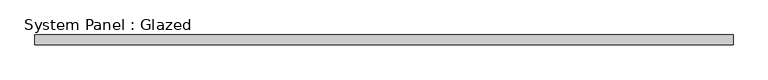
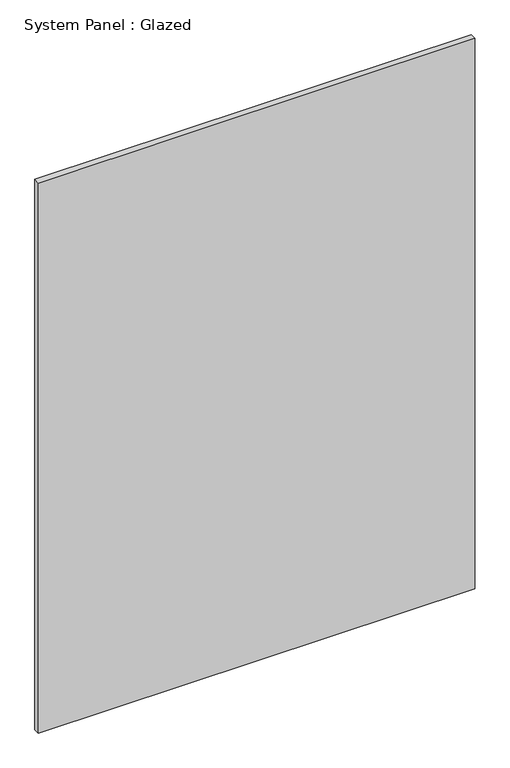
"""IFC4 building model written with IfcOpenShell, lengths in millimetres: plate geometry, System Panel : Glazed."""

from ifc_helpers import new_model, si_unit, origin, origin_with_axes, place, context, project, spatial, polyline, outline, extrude, source, transform, mapped, element, save


def system_panel_glazed_91d575af(model_context):
    return source(origin(), model_context, "Body", "SweptSolid", [
        extrude(outline(polyline([(877.5, 24.5), (-877.5, 24.5), (-877.5, 49.5), (877.5, 49.5), (877.5, 24.5)])), origin_with_axes(), (0.0, 0.0, 1.0), 2338.4),
    ])


if __name__ == "__main__":
    model = new_model("IFC4")
    model_context = context("Model", 3, world=origin())
    ifc_project = project(units=[si_unit("LENGTHUNIT", "METRE", prefix="MILLI")], contexts=[model_context])
    site = spatial("IfcSite", under=ifc_project)
    building = spatial("IfcBuilding", under=site)
    placement = place(None, origin())
    system_panel_glazed_shape = system_panel_glazed_91d575af(model_context)
    element("IfcPlate", 1, ObjectType="System Panel : Glazed", at=placement, inside=building, context=model_context, shape_type="MappedRepresentation", body=[
        mapped(system_panel_glazed_shape, transform((0.0, 0.0, 0.0), x_axis=(1.0, 0.0, 0.0), y_axis=(0.0, 1.0, 0.0), z_axis=(0.0, 0.0, 1.0))),
    ])
    save(model, "model.ifc")

# Revit data of these elements
# Type "System Panel : Glazed"
#   Construction Type Id = "GSP4R"
#   Analytic Construction = "1/8 in Pilkington single glazing"
#   Visual Light Transmittance = 0.9
#   Solar Heat Gain Coefficient = 0.86
#   Heat Transfer Coefficient (U) = 6.7069 W/(m²·K)
# Element 1 (IfcPlate, "System Panel : Glazed")
#   Materials on its faces: "Glass"
# Materials
#   "Glass": class "Glass", colour RGB 0 128 192, transparency 0.9, Description = "Soda Lime Glass", Cost = 0
